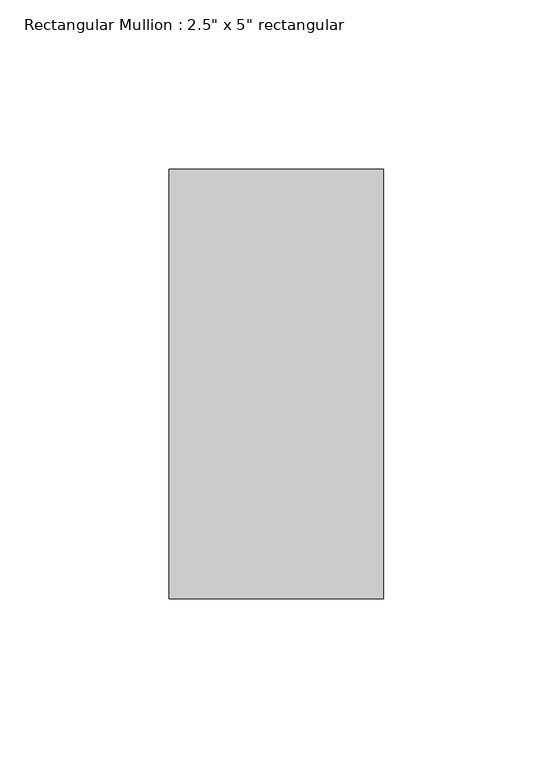
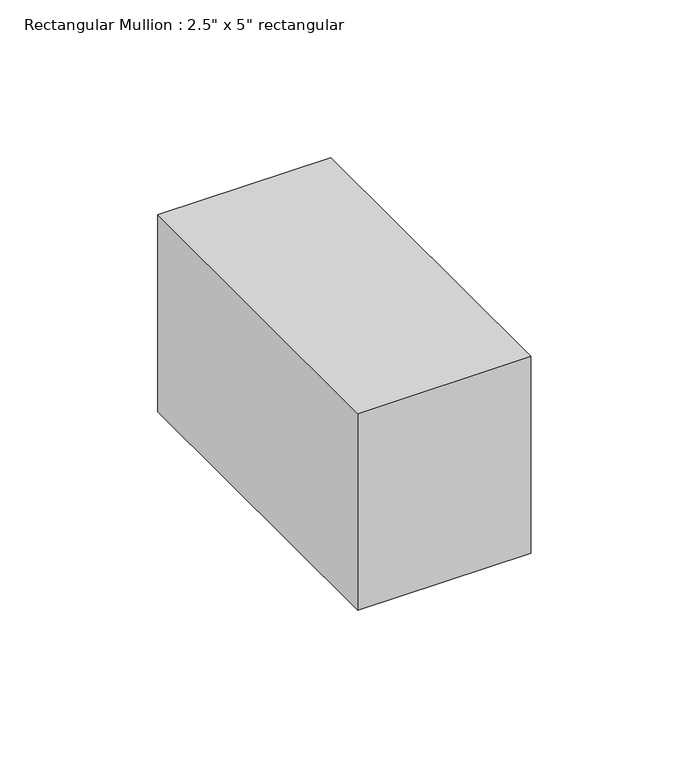
"""IFC4 building model written with IfcOpenShell, lengths in millimetres: member geometry."""

from ifc_helpers import new_model, si_unit, frame, origin, place, context, project, spatial, polyline, outline, extrude, source, transform, mapped, element, save


def member_3d7cb871(model_context):
    return source(origin(), model_context, "Body", "SweptSolid", [
        extrude(outline(polyline([(0.0, 63.5), (0.0, -63.5), (-63.5, -63.5), (-63.5, 63.5), (0.0, 63.5)])), frame((0.0, 0.0, -76.2), z_axis=(0.0, 0.0, 1.0), x_axis=(1.0, 0.0, 0.0)), (0.0, 0.0, 1.0), 76.2),
    ])


if __name__ == "__main__":
    model = new_model("IFC4")
    model_context = context("Model", 3, world=origin())
    ifc_project = project(units=[si_unit("LENGTHUNIT", "METRE", prefix="MILLI")], contexts=[model_context])
    site = spatial("IfcSite", under=ifc_project)
    building = spatial("IfcBuilding", under=site)
    placement = place(None, origin())
    member_shape = member_3d7cb871(model_context)
    element("IfcMember", 1, ObjectType="Rectangular Mullion : 2.5\" x 5\" rectangular", at=placement, inside=building, context=model_context, shape_type="MappedRepresentation", body=[
        mapped(member_shape, transform((0.0, 0.0, 0.0), x_axis=(1.0, 0.0, 0.0), y_axis=(0.0, 1.0, 0.0), z_axis=(0.0, 0.0, 1.0))),
    ])
    save(model, "model.ifc")

# Revit data of these elements
# Type "Rectangular Mullion : 2.5\" x 5\" rectangular"
#   built-in parameter 1007304 = 0.416667 (stored number, unit not read)
#   built-in parameter 1007301 = 0.104167 (stored number, unit not read)
#   built-in parameter 1007300 = 0.104167 (stored number, unit not read)
# Element 1 (IfcMember, "Rectangular Mullion : 2.5\" x 5\" rectangular")
#   Materials on its faces: "Aluminum"
# Materials
#   "Aluminum": class "Metal", colour RGB 247 247 247, transparency 0, Description = "Aluminum 6061", Cost = 0
